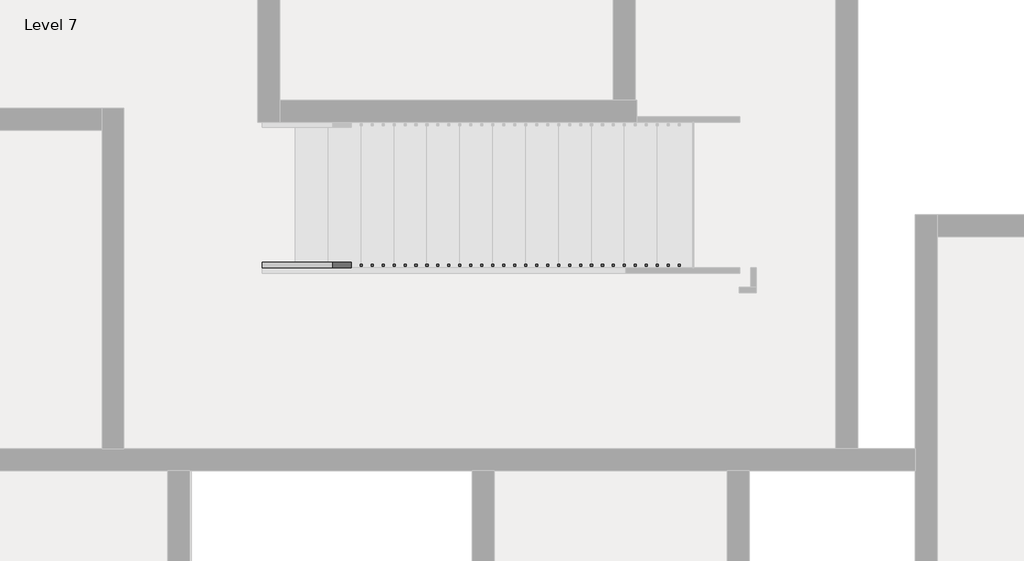
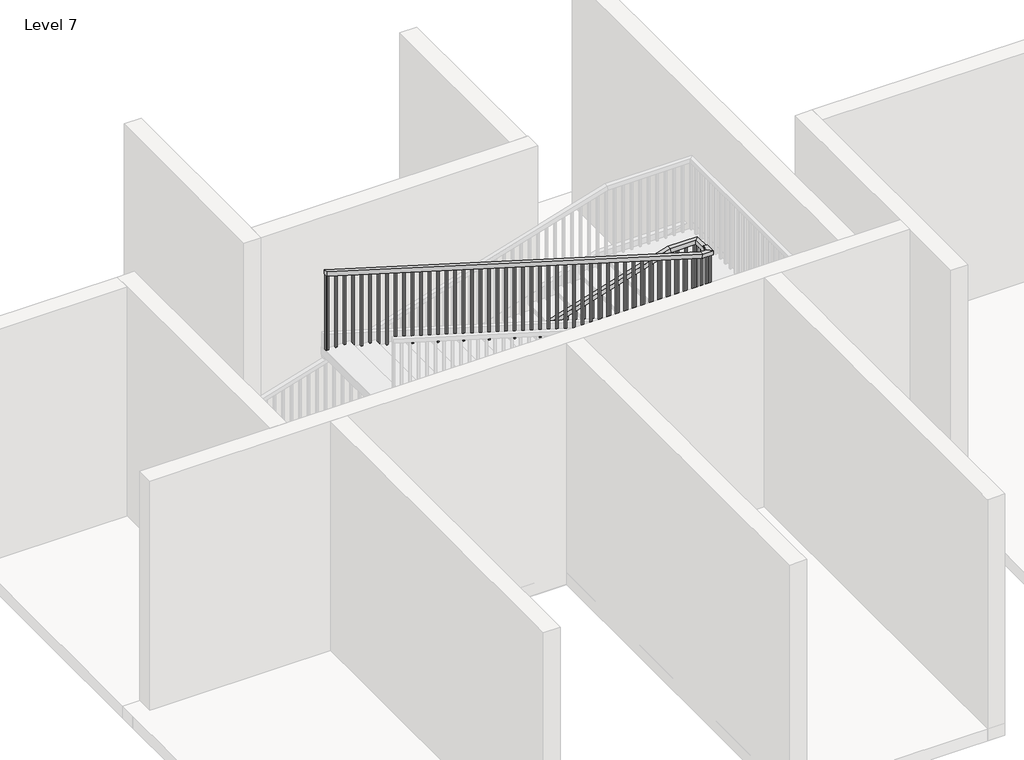
# One storey, part 11 of 14: 1 railing.
"""IFC4 building model written with IfcOpenShell, lengths in millimetres."""

from ifc_helpers import new_model, si_unit, frame, origin, place, context, project, spatial, polyline, outline, extrude, faceted_brep, element, save

model = new_model("IFC4")

# Units and contexts
model_context = context("Model", 3, world=origin())
ifc_project = project(units=[si_unit("LENGTHUNIT", "METRE", prefix="MILLI")], contexts=[model_context])

# Site, building, storey
site = spatial("IfcSite", under=ifc_project)
building = spatial("IfcBuilding", under=site)
storey = spatial("IfcBuildingStorey", under=building, Name="Level 7", Elevation=18288.0)

# Railing
placement = place(None, origin())
element("IfcRailing", 1, ObjectType="Handrail - Rectangular", at=placement, inside=storey, context=model_context, shape_type="SolidModel", body=[
    faceted_brep([(-5254.0891351, 11205.0082924, 19293.84), (-5254.0891351, 11205.0082924, 19240.8032429), (-5254.0891351, 11154.2082924, 19240.8032429), (-5254.0891351, 11154.2082924, 19293.84), (-986.8891351, 11205.0082924, 20574.0), (-979.4332782, 11205.0082924, 20523.2), (-979.4332782, 11154.2082924, 20523.2), (-986.8891351, 11154.2082924, 20574.0), (-631.2891351, 11205.0082924, 20574.0), (-631.2891351, 11205.0082924, 20523.2), (-682.0891351, 11154.2082924, 20523.2), (-682.0891351, 11154.2082924, 20574.0), (-631.2891351, 11001.8082924, 20574.0), (-631.2891351, 10951.0082924, 20523.2), (-682.0891351, 10951.0082924, 20523.2), (-682.0891351, 11001.8082924, 20574.0), (-631.2891351, 11001.8082924, 20596.86), (-631.2891351, 10951.0082924, 20546.06), (-682.0891351, 10951.0082924, 20546.06), (-682.0891351, 11001.8082924, 20596.86), (-631.2891351, 10874.8082924, 20596.86), (-631.2891351, 10874.8082924, 20546.06), (-682.0891351, 10925.6082924, 20546.06), (-682.0891351, 10925.6082924, 20596.86), (-758.2891351, 10874.8082924, 20596.86), (-765.744992, 10874.8082924, 20546.06), (-765.744992, 10925.6082924, 20546.06), (-758.2891351, 10925.6082924, 20596.86), (-5254.0891351, 10874.8082924, 21945.6), (-5254.0891351, 10925.6082924, 21945.6), (-5254.0891351, 10925.6082924, 21892.5632429), (-5254.0891351, 10874.8082924, 21892.5632429)], [[[0, 1, 2, 3]], [[1, 0, 4, 5]], [[2, 1, 5, 6]], [[3, 2, 6, 7]], [[0, 3, 7, 4]], [[5, 4, 8, 9]], [[6, 5, 9, 10]], [[7, 6, 10, 11]], [[4, 7, 11, 8]], [[9, 8, 12, 13]], [[10, 9, 13, 14]], [[11, 10, 14, 15]], [[8, 11, 15, 12]], [[13, 12, 16, 17]], [[14, 13, 17, 18]], [[15, 14, 18, 19]], [[12, 15, 19, 16]], [[17, 16, 20, 21]], [[18, 17, 21, 22]], [[19, 18, 22, 23]], [[16, 19, 23, 20]], [[21, 20, 24, 25]], [[22, 21, 25, 26]], [[23, 22, 26, 27]], [[20, 23, 27, 24]], [[28, 29, 30, 31]], [[25, 24, 28, 31]], [[26, 25, 31, 30]], [[27, 26, 30, 29]], [[24, 27, 29, 28]]]),
    extrude(outline(polyline([(21882.0857429, -5219.1641351), (21887.8007429, -5238.2141351), (20939.76, -5238.2141351), (20939.76, -5219.1641351), (21882.0857429, -5219.1641351)])), frame((0.0, 10890.6832924, 0.0), z_axis=(0.0, 1.0, 0.0), x_axis=(0.0, 0.0, 1.0)), (0.0, 0.0, 1.0), 19.05),
    extrude(outline(polyline([(21851.6057429, -5117.5641351), (21857.3207429, -5136.6141351), (20939.76, -5136.6141351), (20939.76, -5117.5641351), (21851.6057429, -5117.5641351)])), frame((0.0, 10890.6832924, 0.0), z_axis=(0.0, 1.0, 0.0), x_axis=(0.0, 0.0, 1.0)), (0.0, 0.0, 1.0), 19.05),
    extrude(outline(polyline([(21821.1257429, -5015.9641351), (21826.8407429, -5035.0141351), (20939.76, -5035.0141351), (20939.76, -5015.9641351), (21821.1257429, -5015.9641351)])), frame((0.0, 10890.6832924, 0.0), z_axis=(0.0, 1.0, 0.0), x_axis=(0.0, 0.0, 1.0)), (0.0, 0.0, 1.0), 19.05),
    extrude(outline(polyline([(21790.6457429, -4914.3641351), (21796.3607429, -4933.4141351), (20848.32, -4933.4141351), (20848.32, -4914.3641351), (21790.6457429, -4914.3641351)])), frame((0.0, 10890.6832924, 0.0), z_axis=(0.0, 1.0, 0.0), x_axis=(0.0, 0.0, 1.0)), (0.0, 0.0, 1.0), 19.05),
    extrude(outline(polyline([(21760.1657429, -4812.7641351), (21765.8807429, -4831.8141351), (20848.32, -4831.8141351), (20848.32, -4812.7641351), (21760.1657429, -4812.7641351)])), frame((0.0, 10890.6832924, 0.0), z_axis=(0.0, 1.0, 0.0), x_axis=(0.0, 0.0, 1.0)), (0.0, 0.0, 1.0), 19.05),
    extrude(outline(polyline([(21729.6857429, -4711.1641351), (21735.4007429, -4730.2141351), (20848.32, -4730.2141351), (20848.32, -4711.1641351), (21729.6857429, -4711.1641351)])), frame((0.0, 10890.6832924, 0.0), z_axis=(0.0, 1.0, 0.0), x_axis=(0.0, 0.0, 1.0)), (0.0, 0.0, 1.0), 19.05),
    extrude(outline(polyline([(21699.2057429, -4609.5641351), (21704.9207429, -4628.6141351), (20756.88, -4628.6141351), (20756.88, -4609.5641351), (21699.2057429, -4609.5641351)])), frame((0.0, 10890.6832924, 0.0), z_axis=(0.0, 1.0, 0.0), x_axis=(0.0, 0.0, 1.0)), (0.0, 0.0, 1.0), 19.05),
    extrude(outline(polyline([(21668.7257429, -4507.9641351), (21674.4407429, -4527.0141351), (20756.88, -4527.0141351), (20756.88, -4507.9641351), (21668.7257429, -4507.9641351)])), frame((0.0, 10890.6832924, 0.0), z_axis=(0.0, 1.0, 0.0), x_axis=(0.0, 0.0, 1.0)), (0.0, 0.0, 1.0), 19.05),
    extrude(outline(polyline([(21638.2457429, -4406.3641351), (21643.9607429, -4425.4141351), (20756.88, -4425.4141351), (20756.88, -4406.3641351), (21638.2457429, -4406.3641351)])), frame((0.0, 10890.6832924, 0.0), z_axis=(0.0, 1.0, 0.0), x_axis=(0.0, 0.0, 1.0)), (0.0, 0.0, 1.0), 19.05),
    extrude(outline(polyline([(21607.7657429, -4304.7641351), (21613.4807429, -4323.8141351), (20665.44, -4323.8141351), (20665.44, -4304.7641351), (21607.7657429, -4304.7641351)])), frame((0.0, 10890.6832924, 0.0), z_axis=(0.0, 1.0, 0.0), x_axis=(0.0, 0.0, 1.0)), (0.0, 0.0, 1.0), 19.05),
    extrude(outline(polyline([(21577.2857429, -4203.1641351), (21583.0007429, -4222.2141351), (20665.44, -4222.2141351), (20665.44, -4203.1641351), (21577.2857429, -4203.1641351)])), frame((0.0, 10890.6832924, 0.0), z_axis=(0.0, 1.0, 0.0), x_axis=(0.0, 0.0, 1.0)), (0.0, 0.0, 1.0), 19.05),
    extrude(outline(polyline([(21546.8057429, -4101.5641351), (21552.5207429, -4120.6141351), (20665.44, -4120.6141351), (20665.44, -4101.5641351), (21546.8057429, -4101.5641351)])), frame((0.0, 10890.6832924, 0.0), z_axis=(0.0, 1.0, 0.0), x_axis=(0.0, 0.0, 1.0)), (0.0, 0.0, 1.0), 19.05),
    extrude(outline(polyline([(21516.3257429, -3999.9641351), (21522.0407429, -4019.0141351), (20574.0, -4019.0141351), (20574.0, -3999.9641351), (21516.3257429, -3999.9641351)])), frame((0.0, 10890.6832924, 0.0), z_axis=(0.0, 1.0, 0.0), x_axis=(0.0, 0.0, 1.0)), (0.0, 0.0, 1.0), 19.05),
    extrude(outline(polyline([(21485.8457429, -3898.3641351), (21491.5607429, -3917.4141351), (20574.0, -3917.4141351), (20574.0, -3898.3641351), (21485.8457429, -3898.3641351)])), frame((0.0, 10890.6832924, 0.0), z_axis=(0.0, 1.0, 0.0), x_axis=(0.0, 0.0, 1.0)), (0.0, 0.0, 1.0), 19.05),
    extrude(outline(polyline([(21455.3657429, -3796.7641351), (21461.0807429, -3815.8141351), (20574.0, -3815.8141351), (20574.0, -3796.7641351), (21455.3657429, -3796.7641351)])), frame((0.0, 10890.6832924, 0.0), z_axis=(0.0, 1.0, 0.0), x_axis=(0.0, 0.0, 1.0)), (0.0, 0.0, 1.0), 19.05),
    extrude(outline(polyline([(21424.8857429, -3695.1641351), (21430.6007429, -3714.2141351), (20482.56, -3714.2141351), (20482.56, -3695.1641351), (21424.8857429, -3695.1641351)])), frame((0.0, 10890.6832924, 0.0), z_axis=(0.0, 1.0, 0.0), x_axis=(0.0, 0.0, 1.0)), (0.0, 0.0, 1.0), 19.05),
    extrude(outline(polyline([(21394.4057429, -3593.5641351), (21400.1207429, -3612.6141351), (20482.56, -3612.6141351), (20482.56, -3593.5641351), (21394.4057429, -3593.5641351)])), frame((0.0, 10890.6832924, 0.0), z_axis=(0.0, 1.0, 0.0), x_axis=(0.0, 0.0, 1.0)), (0.0, 0.0, 1.0), 19.05),
    extrude(outline(polyline([(21363.9257429, -3491.9641351), (21369.6407429, -3511.0141351), (20482.56, -3511.0141351), (20482.56, -3491.9641351), (21363.9257429, -3491.9641351)])), frame((0.0, 10890.6832924, 0.0), z_axis=(0.0, 1.0, 0.0), x_axis=(0.0, 0.0, 1.0)), (0.0, 0.0, 1.0), 19.05),
    extrude(outline(polyline([(21333.4457429, -3390.3641351), (21339.1607429, -3409.4141351), (20391.12, -3409.4141351), (20391.12, -3390.3641351), (21333.4457429, -3390.3641351)])), frame((0.0, 10890.6832924, 0.0), z_axis=(0.0, 1.0, 0.0), x_axis=(0.0, 0.0, 1.0)), (0.0, 0.0, 1.0), 19.05),
    extrude(outline(polyline([(21302.9657429, -3288.7641351), (21308.6807429, -3307.8141351), (20391.12, -3307.8141351), (20391.12, -3288.7641351), (21302.9657429, -3288.7641351)])), frame((0.0, 10890.6832924, 0.0), z_axis=(0.0, 1.0, 0.0), x_axis=(0.0, 0.0, 1.0)), (0.0, 0.0, 1.0), 19.05),
    extrude(outline(polyline([(21272.4857429, -3187.1641351), (21278.2007429, -3206.2141351), (20391.12, -3206.2141351), (20391.12, -3187.1641351), (21272.4857429, -3187.1641351)])), frame((0.0, 10890.6832924, 0.0), z_axis=(0.0, 1.0, 0.0), x_axis=(0.0, 0.0, 1.0)), (0.0, 0.0, 1.0), 19.05),
    extrude(outline(polyline([(21242.0057429, -3085.5641351), (21247.7207429, -3104.6141351), (20299.68, -3104.6141351), (20299.68, -3085.5641351), (21242.0057429, -3085.5641351)])), frame((0.0, 10890.6832924, 0.0), z_axis=(0.0, 1.0, 0.0), x_axis=(0.0, 0.0, 1.0)), (0.0, 0.0, 1.0), 19.05),
    extrude(outline(polyline([(21211.5257429, -2983.9641351), (21217.2407429, -3003.0141351), (20299.68, -3003.0141351), (20299.68, -2983.9641351), (21211.5257429, -2983.9641351)])), frame((0.0, 10890.6832924, 0.0), z_axis=(0.0, 1.0, 0.0), x_axis=(0.0, 0.0, 1.0)), (0.0, 0.0, 1.0), 19.05),
    extrude(outline(polyline([(21181.0457429, -2882.3641351), (21186.7607429, -2901.4141351), (20299.68, -2901.4141351), (20299.68, -2882.3641351), (21181.0457429, -2882.3641351)])), frame((0.0, 10890.6832924, 0.0), z_axis=(0.0, 1.0, 0.0), x_axis=(0.0, 0.0, 1.0)), (0.0, 0.0, 1.0), 19.05),
    extrude(outline(polyline([(21150.5657429, -2780.7641351), (21156.2807429, -2799.8141351), (20208.24, -2799.8141351), (20208.24, -2780.7641351), (21150.5657429, -2780.7641351)])), frame((0.0, 10890.6832924, 0.0), z_axis=(0.0, 1.0, 0.0), x_axis=(0.0, 0.0, 1.0)), (0.0, 0.0, 1.0), 19.05),
    extrude(outline(polyline([(21120.0857429, -2679.1641351), (21125.8007429, -2698.2141351), (20208.24, -2698.2141351), (20208.24, -2679.1641351), (21120.0857429, -2679.1641351)])), frame((0.0, 10890.6832924, 0.0), z_axis=(0.0, 1.0, 0.0), x_axis=(0.0, 0.0, 1.0)), (0.0, 0.0, 1.0), 19.05),
    extrude(outline(polyline([(21089.6057429, -2577.5641351), (21095.3207429, -2596.6141351), (20208.24, -2596.6141351), (20208.24, -2577.5641351), (21089.6057429, -2577.5641351)])), frame((0.0, 10890.6832924, 0.0), z_axis=(0.0, 1.0, 0.0), x_axis=(0.0, 0.0, 1.0)), (0.0, 0.0, 1.0), 19.05),
    extrude(outline(polyline([(21059.1257429, -2475.9641351), (21064.8407429, -2495.0141351), (20116.8, -2495.0141351), (20116.8, -2475.9641351), (21059.1257429, -2475.9641351)])), frame((0.0, 10890.6832924, 0.0), z_axis=(0.0, 1.0, 0.0), x_axis=(0.0, 0.0, 1.0)), (0.0, 0.0, 1.0), 19.05),
    extrude(outline(polyline([(21028.6457429, -2374.3641351), (21034.3607429, -2393.4141351), (20116.8, -2393.4141351), (20116.8, -2374.3641351), (21028.6457429, -2374.3641351)])), frame((0.0, 10890.6832924, 0.0), z_axis=(0.0, 1.0, 0.0), x_axis=(0.0, 0.0, 1.0)), (0.0, 0.0, 1.0), 19.05),
    extrude(outline(polyline([(20998.1657429, -2272.7641351), (21003.8807429, -2291.8141351), (20116.8, -2291.8141351), (20116.8, -2272.7641351), (20998.1657429, -2272.7641351)])), frame((0.0, 10890.6832924, 0.0), z_axis=(0.0, 1.0, 0.0), x_axis=(0.0, 0.0, 1.0)), (0.0, 0.0, 1.0), 19.05),
    extrude(outline(polyline([(20967.6857429, -2171.1641351), (20973.4007429, -2190.2141351), (20025.36, -2190.2141351), (20025.36, -2171.1641351), (20967.6857429, -2171.1641351)])), frame((0.0, 10890.6832924, 0.0), z_axis=(0.0, 1.0, 0.0), x_axis=(0.0, 0.0, 1.0)), (0.0, 0.0, 1.0), 19.05),
    extrude(outline(polyline([(20937.2057429, -2069.5641351), (20942.9207429, -2088.6141351), (20025.36, -2088.6141351), (20025.36, -2069.5641351), (20937.2057429, -2069.5641351)])), frame((0.0, 10890.6832924, 0.0), z_axis=(0.0, 1.0, 0.0), x_axis=(0.0, 0.0, 1.0)), (0.0, 0.0, 1.0), 19.05),
    extrude(outline(polyline([(20906.7257429, -1967.9641351), (20912.4407429, -1987.0141351), (20025.36, -1987.0141351), (20025.36, -1967.9641351), (20906.7257429, -1967.9641351)])), frame((0.0, 10890.6832924, 0.0), z_axis=(0.0, 1.0, 0.0), x_axis=(0.0, 0.0, 1.0)), (0.0, 0.0, 1.0), 19.05),
    extrude(outline(polyline([(20876.2457429, -1866.3641351), (20881.9607429, -1885.4141351), (19933.92, -1885.4141351), (19933.92, -1866.3641351), (20876.2457429, -1866.3641351)])), frame((0.0, 10890.6832924, 0.0), z_axis=(0.0, 1.0, 0.0), x_axis=(0.0, 0.0, 1.0)), (0.0, 0.0, 1.0), 19.05),
    extrude(outline(polyline([(20845.7657429, -1764.7641351), (20851.4807429, -1783.8141351), (19933.92, -1783.8141351), (19933.92, -1764.7641351), (20845.7657429, -1764.7641351)])), frame((0.0, 10890.6832924, 0.0), z_axis=(0.0, 1.0, 0.0), x_axis=(0.0, 0.0, 1.0)), (0.0, 0.0, 1.0), 19.05),
    extrude(outline(polyline([(20815.2857429, -1663.1641351), (20821.0007429, -1682.2141351), (19933.92, -1682.2141351), (19933.92, -1663.1641351), (20815.2857429, -1663.1641351)])), frame((0.0, 10890.6832924, 0.0), z_axis=(0.0, 1.0, 0.0), x_axis=(0.0, 0.0, 1.0)), (0.0, 0.0, 1.0), 19.05),
    extrude(outline(polyline([(20784.8057429, -1561.5641351), (20790.5207429, -1580.6141351), (19842.48, -1580.6141351), (19842.48, -1561.5641351), (20784.8057429, -1561.5641351)])), frame((0.0, 10890.6832924, 0.0), z_axis=(0.0, 1.0, 0.0), x_axis=(0.0, 0.0, 1.0)), (0.0, 0.0, 1.0), 19.05),
    extrude(outline(polyline([(20754.3257429, -1459.9641351), (20760.0407429, -1479.0141351), (19842.48, -1479.0141351), (19842.48, -1459.9641351), (20754.3257429, -1459.9641351)])), frame((0.0, 10890.6832924, 0.0), z_axis=(0.0, 1.0, 0.0), x_axis=(0.0, 0.0, 1.0)), (0.0, 0.0, 1.0), 19.05),
    extrude(outline(polyline([(20723.8457429, -1358.3641351), (20729.5607429, -1377.4141351), (19842.48, -1377.4141351), (19842.48, -1358.3641351), (20723.8457429, -1358.3641351)])), frame((0.0, 10890.6832924, 0.0), z_axis=(0.0, 1.0, 0.0), x_axis=(0.0, 0.0, 1.0)), (0.0, 0.0, 1.0), 19.05),
    extrude(outline(polyline([(20693.3657429, -1256.7641351), (20699.0807429, -1275.8141351), (19751.04, -1275.8141351), (19751.04, -1256.7641351), (20693.3657429, -1256.7641351)])), frame((0.0, 10890.6832924, 0.0), z_axis=(0.0, 1.0, 0.0), x_axis=(0.0, 0.0, 1.0)), (0.0, 0.0, 1.0), 19.05),
    extrude(outline(polyline([(20662.8857429, -1155.1641351), (20668.6007429, -1174.2141351), (19751.04, -1174.2141351), (19751.04, -1155.1641351), (20662.8857429, -1155.1641351)])), frame((0.0, 10890.6832924, 0.0), z_axis=(0.0, 1.0, 0.0), x_axis=(0.0, 0.0, 1.0)), (0.0, 0.0, 1.0), 19.05),
    extrude(outline(polyline([(20632.4057429, -1053.5641351), (20638.1207429, -1072.6141351), (19751.04, -1072.6141351), (19751.04, -1053.5641351), (20632.4057429, -1053.5641351)])), frame((0.0, 10890.6832924, 0.0), z_axis=(0.0, 1.0, 0.0), x_axis=(0.0, 0.0, 1.0)), (0.0, 0.0, 1.0), 19.05),
    extrude(outline(polyline([(20601.9257429, -951.9641351), (20607.6407429, -971.0141351), (19659.6, -971.0141351), (19659.6, -951.9641351), (20601.9257429, -951.9641351)])), frame((0.0, 10890.6832924, 0.0), z_axis=(0.0, 1.0, 0.0), x_axis=(0.0, 0.0, 1.0)), (0.0, 0.0, 1.0), 19.05),
    extrude(outline(polyline([(20571.4457429, -850.3641351), (20577.1607429, -869.4141351), (19659.6, -869.4141351), (19659.6, -850.3641351), (20571.4457429, -850.3641351)])), frame((0.0, 10890.6832924, 0.0), z_axis=(0.0, 1.0, 0.0), x_axis=(0.0, 0.0, 1.0)), (0.0, 0.0, 1.0), 19.05),
    extrude(outline(polyline([(20540.9657429, -748.7641351), (20546.6807429, -767.8141351), (19659.6, -767.8141351), (19659.6, -748.7641351), (20540.9657429, -748.7641351)])), frame((0.0, 10890.6832924, 0.0), z_axis=(0.0, 1.0, 0.0), x_axis=(0.0, 0.0, 1.0)), (0.0, 0.0, 1.0), 19.05),
    extrude(outline(polyline([(-666.2141351, 10985.9332924), (-647.1641351, 10985.9332924), (-647.1641351, 10966.8832924), (-666.2141351, 10966.8832924), (-666.2141351, 10985.9332924)])), frame((0.0, 0.0, 19659.6), z_axis=(0.0, 0.0, 1.0), x_axis=(1.0, 0.0, 0.0)), (0.0, 0.0, 1.0), 886.46),
    extrude(outline(polyline([(-666.2141351, 11087.5332924), (-647.1641351, 11087.5332924), (-647.1641351, 11068.4832924), (-666.2141351, 11068.4832924), (-666.2141351, 11087.5332924)])), frame((0.0, 0.0, 19659.6), z_axis=(0.0, 0.0, 1.0), x_axis=(1.0, 0.0, 0.0)), (0.0, 0.0, 1.0), 863.6),
    extrude(outline(polyline([(-691.6141351, 11170.0832924), (-691.6141351, 11189.1332924), (-672.5641351, 11189.1332924), (-672.5641351, 11170.0832924), (-691.6141351, 11170.0832924)])), frame((0.0, 0.0, 19659.6), z_axis=(0.0, 0.0, 1.0), x_axis=(1.0, 0.0, 0.0)), (0.0, 0.0, 1.0), 863.6),
    extrude(outline(polyline([(-793.2141351, 11170.0832924), (-793.2141351, 11189.1332924), (-774.1641351, 11189.1332924), (-774.1641351, 11170.0832924), (-793.2141351, 11170.0832924)])), frame((0.0, 0.0, 19659.6), z_axis=(0.0, 0.0, 1.0), x_axis=(1.0, 0.0, 0.0)), (0.0, 0.0, 1.0), 863.6),
    extrude(outline(polyline([(-894.8141351, 11170.0832924), (-894.8141351, 11189.1332924), (-875.7641351, 11189.1332924), (-875.7641351, 11170.0832924), (-894.8141351, 11170.0832924)])), frame((0.0, 0.0, 19659.6), z_axis=(0.0, 0.0, 1.0), x_axis=(1.0, 0.0, 0.0)), (0.0, 0.0, 1.0), 863.6),
    extrude(outline(polyline([(20523.8207429, -977.3641351), (20518.1057429, -996.4141351), (19659.6, -996.4141351), (19659.6, -977.3641351), (20523.8207429, -977.3641351)])), frame((0.0, 11170.0832924, 0.0), z_axis=(0.0, 1.0, 0.0), x_axis=(0.0, 0.0, 1.0)), (0.0, 0.0, 1.0), 19.05),
    extrude(outline(polyline([(20493.3407429, -1078.9641351), (20487.6257429, -1098.0141351), (19568.16, -1098.0141351), (19568.16, -1078.9641351), (20493.3407429, -1078.9641351)])), frame((0.0, 11170.0832924, 0.0), z_axis=(0.0, 1.0, 0.0), x_axis=(0.0, 0.0, 1.0)), (0.0, 0.0, 1.0), 19.05),
    extrude(outline(polyline([(20462.8607429, -1180.5641351), (20457.1457429, -1199.6141351), (19568.16, -1199.6141351), (19568.16, -1180.5641351), (20462.8607429, -1180.5641351)])), frame((0.0, 11170.0832924, 0.0), z_axis=(0.0, 1.0, 0.0), x_axis=(0.0, 0.0, 1.0)), (0.0, 0.0, 1.0), 19.05),
    extrude(outline(polyline([(20432.3807429, -1282.1641351), (20426.6657429, -1301.2141351), (19568.16, -1301.2141351), (19568.16, -1282.1641351), (20432.3807429, -1282.1641351)])), frame((0.0, 11170.0832924, 0.0), z_axis=(0.0, 1.0, 0.0), x_axis=(0.0, 0.0, 1.0)), (0.0, 0.0, 1.0), 19.05),
    extrude(outline(polyline([(20401.9007429, -1383.7641351), (20396.1857429, -1402.8141351), (19476.72, -1402.8141351), (19476.72, -1383.7641351), (20401.9007429, -1383.7641351)])), frame((0.0, 11170.0832924, 0.0), z_axis=(0.0, 1.0, 0.0), x_axis=(0.0, 0.0, 1.0)), (0.0, 0.0, 1.0), 19.05),
    extrude(outline(polyline([(20371.4207429, -1485.3641351), (20365.7057429, -1504.4141351), (19476.72, -1504.4141351), (19476.72, -1485.3641351), (20371.4207429, -1485.3641351)])), frame((0.0, 11170.0832924, 0.0), z_axis=(0.0, 1.0, 0.0), x_axis=(0.0, 0.0, 1.0)), (0.0, 0.0, 1.0), 19.05),
    extrude(outline(polyline([(20340.9407429, -1586.9641351), (20335.2257429, -1606.0141351), (19476.72, -1606.0141351), (19476.72, -1586.9641351), (20340.9407429, -1586.9641351)])), frame((0.0, 11170.0832924, 0.0), z_axis=(0.0, 1.0, 0.0), x_axis=(0.0, 0.0, 1.0)), (0.0, 0.0, 1.0), 19.05),
    extrude(outline(polyline([(20310.4607429, -1688.5641351), (20304.7457429, -1707.6141351), (19385.28, -1707.6141351), (19385.28, -1688.5641351), (20310.4607429, -1688.5641351)])), frame((0.0, 11170.0832924, 0.0), z_axis=(0.0, 1.0, 0.0), x_axis=(0.0, 0.0, 1.0)), (0.0, 0.0, 1.0), 19.05),
    extrude(outline(polyline([(20279.9807429, -1790.1641351), (20274.2657429, -1809.2141351), (19385.28, -1809.2141351), (19385.28, -1790.1641351), (20279.9807429, -1790.1641351)])), frame((0.0, 11170.0832924, 0.0), z_axis=(0.0, 1.0, 0.0), x_axis=(0.0, 0.0, 1.0)), (0.0, 0.0, 1.0), 19.05),
    extrude(outline(polyline([(20249.5007429, -1891.7641351), (20243.7857429, -1910.8141351), (19385.28, -1910.8141351), (19385.28, -1891.7641351), (20249.5007429, -1891.7641351)])), frame((0.0, 11170.0832924, 0.0), z_axis=(0.0, 1.0, 0.0), x_axis=(0.0, 0.0, 1.0)), (0.0, 0.0, 1.0), 19.05),
    extrude(outline(polyline([(20219.0207429, -1993.3641351), (20213.3057429, -2012.4141351), (19293.84, -2012.4141351), (19293.84, -1993.3641351), (20219.0207429, -1993.3641351)])), frame((0.0, 11170.0832924, 0.0), z_axis=(0.0, 1.0, 0.0), x_axis=(0.0, 0.0, 1.0)), (0.0, 0.0, 1.0), 19.05),
    extrude(outline(polyline([(20188.5407429, -2094.9641351), (20182.8257429, -2114.0141351), (19293.84, -2114.0141351), (19293.84, -2094.9641351), (20188.5407429, -2094.9641351)])), frame((0.0, 11170.0832924, 0.0), z_axis=(0.0, 1.0, 0.0), x_axis=(0.0, 0.0, 1.0)), (0.0, 0.0, 1.0), 19.05),
    extrude(outline(polyline([(20158.0607429, -2196.5641351), (20152.3457429, -2215.6141351), (19293.84, -2215.6141351), (19293.84, -2196.5641351), (20158.0607429, -2196.5641351)])), frame((0.0, 11170.0832924, 0.0), z_axis=(0.0, 1.0, 0.0), x_axis=(0.0, 0.0, 1.0)), (0.0, 0.0, 1.0), 19.05),
    extrude(outline(polyline([(20127.5807429, -2298.1641351), (20121.8657429, -2317.2141351), (19202.4, -2317.2141351), (19202.4, -2298.1641351), (20127.5807429, -2298.1641351)])), frame((0.0, 11170.0832924, 0.0), z_axis=(0.0, 1.0, 0.0), x_axis=(0.0, 0.0, 1.0)), (0.0, 0.0, 1.0), 19.05),
    extrude(outline(polyline([(20097.1007429, -2399.7641351), (20091.3857429, -2418.8141351), (19202.4, -2418.8141351), (19202.4, -2399.7641351), (20097.1007429, -2399.7641351)])), frame((0.0, 11170.0832924, 0.0), z_axis=(0.0, 1.0, 0.0), x_axis=(0.0, 0.0, 1.0)), (0.0, 0.0, 1.0), 19.05),
    extrude(outline(polyline([(20066.6207429, -2501.3641351), (20060.9057429, -2520.4141351), (19202.4, -2520.4141351), (19202.4, -2501.3641351), (20066.6207429, -2501.3641351)])), frame((0.0, 11170.0832924, 0.0), z_axis=(0.0, 1.0, 0.0), x_axis=(0.0, 0.0, 1.0)), (0.0, 0.0, 1.0), 19.05),
    extrude(outline(polyline([(20036.1407429, -2602.9641351), (20030.4257429, -2622.0141351), (19110.96, -2622.0141351), (19110.96, -2602.9641351), (20036.1407429, -2602.9641351)])), frame((0.0, 11170.0832924, 0.0), z_axis=(0.0, 1.0, 0.0), x_axis=(0.0, 0.0, 1.0)), (0.0, 0.0, 1.0), 19.05),
    extrude(outline(polyline([(20005.6607429, -2704.5641351), (19999.9457429, -2723.6141351), (19110.96, -2723.6141351), (19110.96, -2704.5641351), (20005.6607429, -2704.5641351)])), frame((0.0, 11170.0832924, 0.0), z_axis=(0.0, 1.0, 0.0), x_axis=(0.0, 0.0, 1.0)), (0.0, 0.0, 1.0), 19.05),
    extrude(outline(polyline([(19975.1807429, -2806.1641351), (19969.4657429, -2825.2141351), (19110.96, -2825.2141351), (19110.96, -2806.1641351), (19975.1807429, -2806.1641351)])), frame((0.0, 11170.0832924, 0.0), z_axis=(0.0, 1.0, 0.0), x_axis=(0.0, 0.0, 1.0)), (0.0, 0.0, 1.0), 19.05),
    extrude(outline(polyline([(19944.7007429, -2907.7641351), (19938.9857429, -2926.8141351), (19019.52, -2926.8141351), (19019.52, -2907.7641351), (19944.7007429, -2907.7641351)])), frame((0.0, 11170.0832924, 0.0), z_axis=(0.0, 1.0, 0.0), x_axis=(0.0, 0.0, 1.0)), (0.0, 0.0, 1.0), 19.05),
    extrude(outline(polyline([(19914.2207429, -3009.3641351), (19908.5057429, -3028.4141351), (19019.52, -3028.4141351), (19019.52, -3009.3641351), (19914.2207429, -3009.3641351)])), frame((0.0, 11170.0832924, 0.0), z_axis=(0.0, 1.0, 0.0), x_axis=(0.0, 0.0, 1.0)), (0.0, 0.0, 1.0), 19.05),
    extrude(outline(polyline([(19883.7407429, -3110.9641351), (19878.0257429, -3130.0141351), (19019.52, -3130.0141351), (19019.52, -3110.9641351), (19883.7407429, -3110.9641351)])), frame((0.0, 11170.0832924, 0.0), z_axis=(0.0, 1.0, 0.0), x_axis=(0.0, 0.0, 1.0)), (0.0, 0.0, 1.0), 19.05),
    extrude(outline(polyline([(19853.2607429, -3212.5641351), (19847.5457429, -3231.6141351), (18928.08, -3231.6141351), (18928.08, -3212.5641351), (19853.2607429, -3212.5641351)])), frame((0.0, 11170.0832924, 0.0), z_axis=(0.0, 1.0, 0.0), x_axis=(0.0, 0.0, 1.0)), (0.0, 0.0, 1.0), 19.05),
    extrude(outline(polyline([(19822.7807429, -3314.1641351), (19817.0657429, -3333.2141351), (18928.08, -3333.2141351), (18928.08, -3314.1641351), (19822.7807429, -3314.1641351)])), frame((0.0, 11170.0832924, 0.0), z_axis=(0.0, 1.0, 0.0), x_axis=(0.0, 0.0, 1.0)), (0.0, 0.0, 1.0), 19.05),
    extrude(outline(polyline([(19792.3007429, -3415.7641351), (19786.5857429, -3434.8141351), (18928.08, -3434.8141351), (18928.08, -3415.7641351), (19792.3007429, -3415.7641351)])), frame((0.0, 11170.0832924, 0.0), z_axis=(0.0, 1.0, 0.0), x_axis=(0.0, 0.0, 1.0)), (0.0, 0.0, 1.0), 19.05),
    extrude(outline(polyline([(19761.8207429, -3517.3641351), (19756.1057429, -3536.4141351), (18836.64, -3536.4141351), (18836.64, -3517.3641351), (19761.8207429, -3517.3641351)])), frame((0.0, 11170.0832924, 0.0), z_axis=(0.0, 1.0, 0.0), x_axis=(0.0, 0.0, 1.0)), (0.0, 0.0, 1.0), 19.05),
    extrude(outline(polyline([(19731.3407429, -3618.9641351), (19725.6257429, -3638.0141351), (18836.64, -3638.0141351), (18836.64, -3618.9641351), (19731.3407429, -3618.9641351)])), frame((0.0, 11170.0832924, 0.0), z_axis=(0.0, 1.0, 0.0), x_axis=(0.0, 0.0, 1.0)), (0.0, 0.0, 1.0), 19.05),
    extrude(outline(polyline([(19700.8607429, -3720.5641351), (19695.1457429, -3739.6141351), (18836.64, -3739.6141351), (18836.64, -3720.5641351), (19700.8607429, -3720.5641351)])), frame((0.0, 11170.0832924, 0.0), z_axis=(0.0, 1.0, 0.0), x_axis=(0.0, 0.0, 1.0)), (0.0, 0.0, 1.0), 19.05),
    extrude(outline(polyline([(19670.3807429, -3822.1641351), (19664.6657429, -3841.2141351), (18745.2, -3841.2141351), (18745.2, -3822.1641351), (19670.3807429, -3822.1641351)])), frame((0.0, 11170.0832924, 0.0), z_axis=(0.0, 1.0, 0.0), x_axis=(0.0, 0.0, 1.0)), (0.0, 0.0, 1.0), 19.05),
    extrude(outline(polyline([(19639.9007429, -3923.7641351), (19634.1857429, -3942.8141351), (18745.2, -3942.8141351), (18745.2, -3923.7641351), (19639.9007429, -3923.7641351)])), frame((0.0, 11170.0832924, 0.0), z_axis=(0.0, 1.0, 0.0), x_axis=(0.0, 0.0, 1.0)), (0.0, 0.0, 1.0), 19.05),
    extrude(outline(polyline([(19609.4207429, -4025.3641351), (19603.7057429, -4044.4141351), (18745.2, -4044.4141351), (18745.2, -4025.3641351), (19609.4207429, -4025.3641351)])), frame((0.0, 11170.0832924, 0.0), z_axis=(0.0, 1.0, 0.0), x_axis=(0.0, 0.0, 1.0)), (0.0, 0.0, 1.0), 19.05),
    extrude(outline(polyline([(19578.9407429, -4126.9641351), (19573.2257429, -4146.0141351), (18653.76, -4146.0141351), (18653.76, -4126.9641351), (19578.9407429, -4126.9641351)])), frame((0.0, 11170.0832924, 0.0), z_axis=(0.0, 1.0, 0.0), x_axis=(0.0, 0.0, 1.0)), (0.0, 0.0, 1.0), 19.05),
    extrude(outline(polyline([(19548.4607429, -4228.5641351), (19542.7457429, -4247.6141351), (18653.76, -4247.6141351), (18653.76, -4228.5641351), (19548.4607429, -4228.5641351)])), frame((0.0, 11170.0832924, 0.0), z_axis=(0.0, 1.0, 0.0), x_axis=(0.0, 0.0, 1.0)), (0.0, 0.0, 1.0), 19.05),
    extrude(outline(polyline([(19517.9807429, -4330.1641351), (19512.2657429, -4349.2141351), (18653.76, -4349.2141351), (18653.76, -4330.1641351), (19517.9807429, -4330.1641351)])), frame((0.0, 11170.0832924, 0.0), z_axis=(0.0, 1.0, 0.0), x_axis=(0.0, 0.0, 1.0)), (0.0, 0.0, 1.0), 19.05),
    extrude(outline(polyline([(19487.5007429, -4431.7641351), (19481.7857429, -4450.8141351), (18562.32, -4450.8141351), (18562.32, -4431.7641351), (19487.5007429, -4431.7641351)])), frame((0.0, 11170.0832924, 0.0), z_axis=(0.0, 1.0, 0.0), x_axis=(0.0, 0.0, 1.0)), (0.0, 0.0, 1.0), 19.05),
    extrude(outline(polyline([(19457.0207429, -4533.3641351), (19451.3057429, -4552.4141351), (18562.32, -4552.4141351), (18562.32, -4533.3641351), (19457.0207429, -4533.3641351)])), frame((0.0, 11170.0832924, 0.0), z_axis=(0.0, 1.0, 0.0), x_axis=(0.0, 0.0, 1.0)), (0.0, 0.0, 1.0), 19.05),
    extrude(outline(polyline([(19426.5407429, -4634.9641351), (19420.8257429, -4654.0141351), (18562.32, -4654.0141351), (18562.32, -4634.9641351), (19426.5407429, -4634.9641351)])), frame((0.0, 11170.0832924, 0.0), z_axis=(0.0, 1.0, 0.0), x_axis=(0.0, 0.0, 1.0)), (0.0, 0.0, 1.0), 19.05),
    extrude(outline(polyline([(19396.0607429, -4736.5641351), (19390.3457429, -4755.6141351), (18470.88, -4755.6141351), (18470.88, -4736.5641351), (19396.0607429, -4736.5641351)])), frame((0.0, 11170.0832924, 0.0), z_axis=(0.0, 1.0, 0.0), x_axis=(0.0, 0.0, 1.0)), (0.0, 0.0, 1.0), 19.05),
    extrude(outline(polyline([(19365.5807429, -4838.1641351), (19359.8657429, -4857.2141351), (18470.88, -4857.2141351), (18470.88, -4838.1641351), (19365.5807429, -4838.1641351)])), frame((0.0, 11170.0832924, 0.0), z_axis=(0.0, 1.0, 0.0), x_axis=(0.0, 0.0, 1.0)), (0.0, 0.0, 1.0), 19.05),
    extrude(outline(polyline([(19335.1007429, -4939.7641351), (19329.3857429, -4958.8141351), (18470.88, -4958.8141351), (18470.88, -4939.7641351), (19335.1007429, -4939.7641351)])), frame((0.0, 11170.0832924, 0.0), z_axis=(0.0, 1.0, 0.0), x_axis=(0.0, 0.0, 1.0)), (0.0, 0.0, 1.0), 19.05),
    extrude(outline(polyline([(19304.6207429, -5041.3641351), (19298.9057429, -5060.4141351), (18379.44, -5060.4141351), (18379.44, -5041.3641351), (19304.6207429, -5041.3641351)])), frame((0.0, 11170.0832924, 0.0), z_axis=(0.0, 1.0, 0.0), x_axis=(0.0, 0.0, 1.0)), (0.0, 0.0, 1.0), 19.05),
    extrude(outline(polyline([(19274.1407429, -5142.9641351), (19268.4257429, -5162.0141351), (18379.44, -5162.0141351), (18379.44, -5142.9641351), (19274.1407429, -5142.9641351)])), frame((0.0, 11170.0832924, 0.0), z_axis=(0.0, 1.0, 0.0), x_axis=(0.0, 0.0, 1.0)), (0.0, 0.0, 1.0), 19.05),
    extrude(outline(polyline([(-666.2141351, 10909.7332924), (-647.1641351, 10909.7332924), (-647.1641351, 10890.6832924), (-666.2141351, 10890.6832924), (-666.2141351, 10909.7332924)])), frame((0.0, 0.0, 19659.6), z_axis=(0.0, 0.0, 1.0), x_axis=(1.0, 0.0, 0.0)), (0.0, 0.0, 1.0), 886.46),
    extrude(outline(polyline([(-666.2141351, 11170.0832924), (-666.2141351, 11189.1332924), (-647.1641351, 11189.1332924), (-647.1641351, 11170.0832924), (-666.2141351, 11170.0832924)])), frame((0.0, 0.0, 19659.6), z_axis=(0.0, 0.0, 1.0), x_axis=(1.0, 0.0, 0.0)), (0.0, 0.0, 1.0), 863.6),
    extrude(outline(polyline([(21886.8482429, -5235.0391351), (21892.5632429, -5254.0891351), (20939.76, -5254.0891351), (20939.76, -5235.0391351), (21886.8482429, -5235.0391351)])), frame((0.0, 10890.6832924, 0.0), z_axis=(0.0, 1.0, 0.0), x_axis=(0.0, 0.0, 1.0)), (0.0, 0.0, 1.0), 19.05),
    extrude(outline(polyline([(19246.5182429, -5235.0391351), (19240.8032429, -5254.0891351), (18379.44, -5254.0891351), (18379.44, -5235.0391351), (19246.5182429, -5235.0391351)])), frame((0.0, 11170.0832924, 0.0), z_axis=(0.0, 1.0, 0.0), x_axis=(0.0, 0.0, 1.0)), (0.0, 0.0, 1.0), 19.05),
])

save(model, "model.ifc")

# Revit data of these elements
# Type "Handrail - Rectangular"
#   Assembly Code = "C2010400"
#   built-in parameter 1008612 = 0.0416667 (stored number, unit not read)
#   built-in parameter 1008611 = 0.0416667 (stored number, unit not read)
#   built-in parameter 1008609 = 0.333333 (stored number, unit not read)
#   built-in parameter 1008604 = 0.166667 (stored number, unit not read)
#   built-in parameter 1008603 = 0.166667 (stored number, unit not read)
#   Railing Height = 3' - 0"
#   built-in parameter 1008630 = 2
#   built-in parameter 1008610 = 2
#   built-in parameter 1008618 = Baluster - Square : 3/4"
# Element 1 (IfcRailing, "Handrail - Rectangular")
#   Phase Created = New Construction
